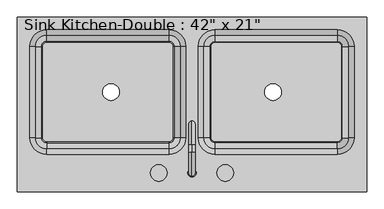
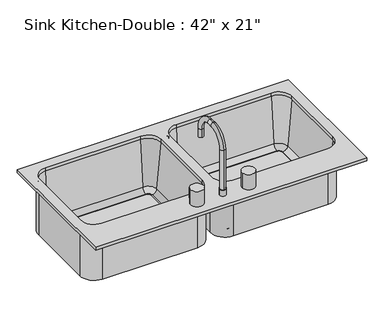
"""IFC4 building model written with IfcOpenShell, lengths in millimetres: flow terminal geometry."""

from ifc_helpers import new_model, si_unit, point, frame, frame_2d, origin, place, context, project, spatial, polyline, circle_curve, ellipse_curve, trimmed, segment, composite_curve, outline, extrude, source, transform, mapped, element, save
from ifc_brep_helpers import plane_surface, cylinder_surface, revolved_surface, advanced_brep


def flow_terminal_7482ecd1(model_context):
    return source(origin(), model_context, "Body", "SolidModel", [
        advanced_brep(
        [(2.9892406, -211.8954011, 927.1), (28.3892406, -211.8954011, 927.1), (15.6892406, -221.4204011, 1114.425), (15.6892406, -221.4204011, 952.5), (15.6892406, -202.3704011, 952.5), (15.6892406, -202.3704011, 1114.425), (15.6892406, -148.3954011, 1168.4), (15.6892406, -148.3954011, 1187.45), (15.6892406, -126.1704011, 1168.4), (15.6892406, -126.1704011, 1187.45), (15.6892406, -72.1954011, 1114.425), (15.6892406, -53.1454011, 1114.425), (15.6892406, -53.1454011, 1079.5), (15.6892406, -72.1954011, 1079.5), (2.9892406, -211.8954011, 952.5), (28.3892406, -211.8954011, 952.5)],
        [
            (0, 1, circle_curve(frame((15.6892406, -211.8954011, 927.1), z_axis=(0.0, 0.0, -1.0), x_axis=(1.0, 0.0, 0.0)), 12.7)),
            (1, 0, circle_curve(frame((15.6892406, -211.8954011, 927.1), z_axis=(0.0, 0.0, -1.0), x_axis=(1.0, 0.0, 0.0)), 12.7)),
            (2, 3),
            (3, 4, circle_curve(frame((15.6892406, -211.8954011, 952.5), z_axis=(0.0, 0.0, 1.0), x_axis=(0.0, 1.0, 0.0)), 9.525)),
            (4, 5),
            (5, 2, circle_curve(frame((15.6892406, -211.8954011, 1114.425), z_axis=(0.0, 0.0, -1.0), x_axis=(0.0, 1.0, 0.0)), 9.525)),
            (4, 3, circle_curve(frame((15.6892406, -211.8954011, 952.5), z_axis=(0.0, 0.0, 1.0), x_axis=(0.0, 1.0, 0.0)), 9.525)),
            (2, 5, circle_curve(frame((15.6892406, -211.8954011, 1114.425), z_axis=(0.0, 0.0, -1.0), x_axis=(0.0, 1.0, 0.0)), 9.525)),
            (5, 6, circle_curve(frame((15.6892406, -148.3954011, 1114.425), z_axis=(-1.0, 0.0, 0.0), x_axis=(0.0, -1.0, 0.0)), 53.975)),
            (6, 7, circle_curve(frame((15.6892406, -148.3954011, 1177.925), z_axis=(0.0, -1.0, 0.0), x_axis=(0.0, 0.0, -1.0)), 9.525)),
            (7, 2, circle_curve(frame((15.6892406, -148.3954011, 1114.425), z_axis=(1.0, 0.0, 0.0), x_axis=(0.0, -1.0, 0.0)), 73.025)),
            (7, 6, circle_curve(frame((15.6892406, -148.3954011, 1177.925), z_axis=(0.0, -1.0, 0.0), x_axis=(0.0, 0.0, -1.0)), 9.525)),
            (6, 8),
            (8, 9, circle_curve(frame((15.6892406, -126.1704011, 1177.925), z_axis=(0.0, -1.0, 0.0), x_axis=(0.0, 0.0, -1.0)), 9.525)),
            (9, 7),
            (9, 8, circle_curve(frame((15.6892406, -126.1704011, 1177.925), z_axis=(0.0, -1.0, 0.0), x_axis=(0.0, 0.0, -1.0)), 9.525)),
            (8, 10, circle_curve(frame((15.6892406, -126.1704011, 1114.425), z_axis=(-1.0, 0.0, 0.0), x_axis=(0.0, 0.0, 1.0)), 53.975)),
            (10, 11, circle_curve(frame((15.6892406, -62.6704011, 1114.425), z_axis=(0.0, 0.0, 1.0), x_axis=(0.0, -1.0, 0.0)), 9.525)),
            (11, 9, circle_curve(frame((15.6892406, -126.1704011, 1114.425), z_axis=(1.0, 0.0, 0.0), x_axis=(0.0, 0.0, 1.0)), 73.025)),
            (11, 10, circle_curve(frame((15.6892406, -62.6704011, 1114.425), z_axis=(0.0, 0.0, 1.0), x_axis=(0.0, -1.0, 0.0)), 9.525)),
            (12, 13, circle_curve(frame((15.6892406, -62.6704011, 1079.5), z_axis=(0.0, 0.0, -1.0), x_axis=(0.0, -1.0, 0.0)), 9.525)),
            (13, 12, circle_curve(frame((15.6892406, -62.6704011, 1079.5), z_axis=(0.0, 0.0, -1.0), x_axis=(0.0, -1.0, 0.0)), 9.525)),
            (10, 13),
            (12, 11),
            (14, 15, circle_curve(frame((15.6892406, -211.8954011, 952.5), z_axis=(0.0, 0.0, 1.0), x_axis=(1.0, 0.0, 0.0)), 12.7)),
            (15, 14, circle_curve(frame((15.6892406, -211.8954011, 952.5), z_axis=(0.0, 0.0, 1.0), x_axis=(1.0, 0.0, 0.0)), 12.7)),
            (15, 1),
            (0, 14),
        ],
        [
            plane_surface(frame((15.6892406, -202.3704011, 927.1), z_axis=(0.0, 0.0, -1.0), x_axis=(1.0, 0.0, 0.0))),
            cylinder_surface(frame((15.6892406, -211.8954011, 927.1), z_axis=(0.0, 0.0, -1.0), x_axis=(0.0, 1.0, 0.0)), 9.525),
            revolved_surface(trimmed(ellipse_curve(frame((15.6892406, -211.8954011, 1114.425), z_axis=(0.0, 0.0, 1.0), x_axis=(0.0, 1.0, 0.0)), 9.525, 9.525), [point((15.6892406, -221.4204011, 1114.425))], [point((15.6892406, -202.3704011, 1114.425))], True, "CARTESIAN"), (15.6892406, -148.3954011, 1114.425), (1.0, 0.0, 0.0)),
            revolved_surface(trimmed(ellipse_curve(frame((15.6892406, -211.8954011, 1114.425), z_axis=(0.0, 0.0, 1.0), x_axis=(0.0, 1.0, 0.0)), 9.525, 9.525), [point((15.6892406, -202.3704011, 1114.425))], [point((15.6892406, -221.4204011, 1114.425))], True, "CARTESIAN"), (15.6892406, -148.3954011, 1114.425), (1.0, 0.0, 0.0)),
            cylinder_surface(frame((15.6892406, -148.3954011, 1177.925), z_axis=(0.0, -1.0, 0.0), x_axis=(0.0, 0.0, -1.0)), 9.525),
            revolved_surface(trimmed(ellipse_curve(frame((15.6892406, -126.1704011, 1177.925), z_axis=(0.0, 1.0, 0.0), x_axis=(0.0, 0.0, -1.0)), 9.525, 9.525), [point((15.6892406, -126.1704011, 1187.45))], [point((15.6892406, -126.1704011, 1168.4))], True, "CARTESIAN"), (15.6892406, -126.1704011, 1114.425), (1.0, 0.0, 0.0)),
            revolved_surface(trimmed(ellipse_curve(frame((15.6892406, -126.1704011, 1177.925), z_axis=(0.0, 1.0, 0.0), x_axis=(0.0, 0.0, -1.0)), 9.525, 9.525), [point((15.6892406, -126.1704011, 1168.4))], [point((15.6892406, -126.1704011, 1187.45))], True, "CARTESIAN"), (15.6892406, -126.1704011, 1114.425), (1.0, 0.0, 0.0)),
            plane_surface(frame((15.6892406, -53.1454011, 1079.5), z_axis=(0.0, 0.0, -1.0), x_axis=(-1.0, 0.0, 0.0))),
            cylinder_surface(frame((15.6892406, -62.6704011, 1114.425), z_axis=(0.0, 0.0, 1.0), x_axis=(0.0, -1.0, 0.0)), 9.525),
            plane_surface(frame((28.3892406, -211.8954011, 952.5), z_axis=(0.0, 0.0, 1.0), x_axis=(0.0, -1.0, 0.0))),
            cylinder_surface(frame((15.6892406, -211.8954011, 927.1), z_axis=(0.0, 0.0, 1.0), x_axis=(1.0, 0.0, 0.0)), 12.7),
        ],
        [
            (0, [[1, 2]]),
            (1, [[3, 4, 5, 6]]),
            (1, [[-5, 7, -3, 8]]),
            (2, [[9, 10, 11, -6]]),
            (3, [[-11, 12, -9, -8]]),
            (4, [[13, 14, 15, -10]]),
            (4, [[-15, 16, -13, -12]]),
            (5, [[17, 18, 19, -14]]),
            (6, [[-19, 20, -17, -16]]),
            (7, [[21, 22]]),
            (8, [[23, -21, 24, -18]]),
            (8, [[-24, -22, -23, -20]]),
            (9, [[25, 26], [-7, -4]]),
            (10, [[27, -1, 28, -26]]),
            (10, [[-28, -2, -27, -25]]),
        ],
    ),
        advanced_brep(
        [(549.0892406, -269.0454011, 927.1), (549.0892406, 264.3545989, 927.1), (-517.7107594, 264.3545989, 927.1), (-517.7107594, -269.0454011, 927.1), (-54.1607594, -154.7454011, 927.1), (-428.8107594, -154.7454011, 927.1), (-479.6107594, -103.9454011, 927.1), (-479.6107594, 175.4545989, 927.1), (-428.8107594, 226.2545989, 927.1), (-54.1607594, 226.2545989, 927.1), (-3.3607594, 175.4545989, 927.1), (-3.3607594, -103.9454011, 927.1), (85.5392406, 226.2545989, 927.1), (460.1892406, 226.2545989, 927.1), (510.9892406, 175.4545989, 927.1), (510.9892406, -103.9454011, 927.1), (460.1892406, -154.7454011, 927.1), (85.5392406, -154.7454011, 927.1), (34.7392406, -103.9454011, 927.1), (34.7392406, 175.4545989, 927.1), (549.0892406, -269.0454011, 914.4), (-517.7107594, -269.0454011, 914.4), (-517.7107594, 264.3545989, 914.4), (549.0892406, 264.3545989, 914.4), (85.5392406, -161.0954011, 914.4), (460.1892406, -161.0954011, 914.4), (517.3392406, -103.9454011, 914.4), (517.3392406, 175.4545989, 914.4), (460.1892406, 232.6045989, 914.4), (85.5392406, 232.6045989, 914.4), (28.3892406, 175.4545989, 914.4), (28.3892406, -103.9454011, 914.4), (2.9892406, -103.9454011, 914.4), (2.9892406, 175.4545989, 914.4), (-54.1607594, 232.6045989, 914.4), (-428.8107594, 232.6045989, 914.4), (-485.9607594, 175.4545989, 914.4), (-485.9607594, -103.9454011, 914.4), (-428.8107594, -161.0954011, 914.4), (-54.1607594, -161.0954011, 914.4), (-3.3607594, -103.9454011, 914.4), (-54.1607594, -154.7454011, 914.4), (-3.3607594, 175.4545989, 914.4), (-54.1607594, 226.2545989, 914.4), (-428.8107594, 226.2545989, 914.4), (-479.6107594, 175.4545989, 914.4), (-479.6107594, -103.9454011, 914.4), (-428.8107594, -154.7454011, 914.4), (34.7392406, 175.4545989, 914.4), (85.5392406, 226.2545989, 914.4), (34.7392406, -103.9454011, 914.4), (85.5392406, -154.7454011, 914.4), (460.1892406, -154.7454011, 914.4), (510.9892406, -103.9454011, 914.4), (510.9892406, 175.4545989, 914.4), (460.1892406, 226.2545989, 914.4), (2.9892406, -103.9454011, 698.5), (-54.1607594, -161.0954011, 698.5), (-54.1607594, -116.6454011, 698.5), (-41.4607594, -103.9454011, 698.5), (-54.1607594, -116.6454011, 708.025), (-41.4607594, -103.9454011, 708.025), (-54.1607594, -119.2338193, 708.025), (-38.8723412, -103.9454011, 708.025), (-54.1607594, -138.2113283, 725.4146831), (-19.8948322, -103.9454011, 725.4146831), (2.9892406, 175.4545989, 698.5), (-41.4607594, 175.4545989, 698.5), (-41.4607594, 175.4545989, 708.025), (-38.8723412, 175.4545989, 708.025), (-19.8948322, 175.4545989, 725.4146831), (-54.1607594, 232.6045989, 698.5), (-54.1607594, 188.1545989, 698.5), (-54.1607594, 188.1545989, 708.025), (-54.1607594, 190.7430171, 708.025), (-54.1607594, 209.7205261, 725.4146831), (-428.8107594, 232.6045989, 698.5), (-428.8107594, 188.1545989, 698.5), (-428.8107594, 188.1545989, 708.025), (-428.8107594, 190.7430171, 708.025), (-428.8107594, 209.7205261, 725.4146831), (-485.9607594, 175.4545989, 698.5), (-441.5107594, 175.4545989, 698.5), (-441.5107594, 175.4545989, 708.025), (-444.0991776, 175.4545989, 708.025), (-463.0766866, 175.4545989, 725.4146831), (-485.9607594, -103.9454011, 698.5), (-441.5107594, -103.9454011, 698.5), (-441.5107594, -103.9454011, 708.025), (-444.0991776, -103.9454011, 708.025), (-463.0766866, -103.9454011, 725.4146831), (-428.8107594, -161.0954011, 698.5), (-428.8107594, -116.6454011, 698.5), (-428.8107594, -116.6454011, 708.025), (-428.8107594, -119.2338193, 708.025), (-428.8107594, -138.2113283, 725.4146831), (51.2733134, -103.9454011, 725.4146831), (85.5392406, -138.2113283, 725.4146831), (85.5392406, -119.2338193, 708.025), (70.2508224, -103.9454011, 708.025), (85.5392406, -116.6454011, 708.025), (72.8392406, -103.9454011, 708.025), (85.5392406, -116.6454011, 698.5), (72.8392406, -103.9454011, 698.5), (85.5392406, -161.0954011, 698.5), (28.3892406, -103.9454011, 698.5), (51.2733134, 175.4545989, 725.4146831), (70.2508224, 175.4545989, 708.025), (72.8392406, 175.4545989, 708.025), (72.8392406, 175.4545989, 698.5), (28.3892406, 175.4545989, 698.5), (85.5392406, 209.7205261, 725.4146831), (85.5392406, 190.7430171, 708.025), (85.5392406, 188.1545989, 708.025), (85.5392406, 188.1545989, 698.5), (85.5392406, 232.6045989, 698.5), (460.1892406, 209.7205261, 725.4146831), (460.1892406, 190.7430171, 708.025), (460.1892406, 188.1545989, 708.025), (460.1892406, 188.1545989, 698.5), (460.1892406, 232.6045989, 698.5), (494.4551678, 175.4545989, 725.4146831), (475.4776588, 175.4545989, 708.025), (472.8892406, 175.4545989, 708.025), (472.8892406, 175.4545989, 698.5), (517.3392406, 175.4545989, 698.5), (494.4551678, -103.9454011, 725.4146831), (475.4776588, -103.9454011, 708.025), (472.8892406, -103.9454011, 708.025), (472.8892406, -103.9454011, 698.5), (517.3392406, -103.9454011, 698.5), (460.1892406, -138.2113283, 725.4146831), (460.1892406, -119.2338193, 708.025), (460.1892406, -116.6454011, 708.025), (460.1892406, -116.6454011, 698.5), (460.1892406, -161.0954011, 698.5)],
        [
            (0, 1),
            (1, 2),
            (2, 3),
            (3, 0),
            (4, 5),
            (5, 6, circle_curve(frame((-428.8107594, -103.9454011, 927.1), z_axis=(0.0, 0.0, -1.0), x_axis=(1.0, 0.0, 0.0)), 50.8)),
            (6, 7),
            (7, 8, circle_curve(frame((-428.8107594, 175.4545989, 927.1), z_axis=(0.0, 0.0, -1.0), x_axis=(1.0, 0.0, 0.0)), 50.8)),
            (8, 9),
            (9, 10, circle_curve(frame((-54.1607594, 175.4545989, 927.1), z_axis=(0.0, 0.0, -1.0), x_axis=(1.0, 0.0, 0.0)), 50.8)),
            (10, 11),
            (11, 4, circle_curve(frame((-54.1607594, -103.9454011, 927.1), z_axis=(0.0, 0.0, -1.0), x_axis=(1.0, 0.0, 0.0)), 50.8)),
            (12, 13),
            (13, 14, circle_curve(frame((460.1892406, 175.4545989, 927.1), z_axis=(0.0, 0.0, -1.0), x_axis=(1.0, 0.0, 0.0)), 50.8)),
            (14, 15),
            (15, 16, circle_curve(frame((460.1892406, -103.9454011, 927.1), z_axis=(0.0, 0.0, -1.0), x_axis=(1.0, 0.0, 0.0)), 50.8)),
            (16, 17),
            (17, 18, circle_curve(frame((85.5392406, -103.9454011, 927.1), z_axis=(0.0, 0.0, -1.0), x_axis=(1.0, 0.0, 0.0)), 50.8)),
            (18, 19),
            (19, 12, circle_curve(frame((85.5392406, 175.4545989, 927.1), z_axis=(0.0, 0.0, -1.0), x_axis=(1.0, 0.0, 0.0)), 50.8)),
            (20, 21),
            (21, 22),
            (22, 23),
            (23, 20),
            (24, 25),
            (25, 26, circle_curve(frame((460.1892406, -103.9454011, 914.4), z_axis=(0.0, 0.0, 1.0), x_axis=(1.0, 0.0, 0.0)), 57.15)),
            (26, 27),
            (27, 28, circle_curve(frame((460.1892406, 175.4545989, 914.4), z_axis=(0.0, 0.0, 1.0), x_axis=(0.0, 1.0, 0.0)), 57.15)),
            (28, 29),
            (29, 30, circle_curve(frame((85.5392406, 175.4545989, 914.4), z_axis=(0.0, 0.0, 1.0), x_axis=(-1.0, 0.0, 0.0)), 57.15)),
            (30, 31),
            (31, 24, circle_curve(frame((85.5392406, -103.9454011, 914.4), z_axis=(0.0, 0.0, 1.0), x_axis=(0.0, -1.0, 0.0)), 57.15)),
            (32, 33),
            (33, 34, circle_curve(frame((-54.1607594, 175.4545989, 914.4), z_axis=(0.0, 0.0, 1.0), x_axis=(1.0, 0.0, 0.0)), 57.15)),
            (34, 35),
            (35, 36, circle_curve(frame((-428.8107594, 175.4545989, 914.4), z_axis=(0.0, 0.0, 1.0), x_axis=(0.0, 1.0, 0.0)), 57.15)),
            (36, 37),
            (37, 38, circle_curve(frame((-428.8107594, -103.9454011, 914.4), z_axis=(0.0, 0.0, 1.0), x_axis=(-1.0, 0.0, 0.0)), 57.15)),
            (38, 39),
            (39, 32, circle_curve(frame((-54.1607594, -103.9454011, 914.4), z_axis=(0.0, 0.0, 1.0), x_axis=(0.0, -1.0, 0.0)), 57.15)),
            (3, 21),
            (20, 0),
            (2, 22),
            (1, 23),
            (11, 40),
            (40, 41, circle_curve(frame((-54.1607594, -103.9454011, 914.4), z_axis=(0.0, 0.0, -1.0), x_axis=(1.0, 0.0, 0.0)), 50.8)),
            (41, 4),
            (10, 42),
            (42, 40),
            (9, 43),
            (43, 42, circle_curve(frame((-54.1607594, 175.4545989, 914.4), z_axis=(0.0, 0.0, -1.0), x_axis=(1.0, 0.0, 0.0)), 50.8)),
            (8, 44),
            (44, 43),
            (7, 45),
            (45, 44, circle_curve(frame((-428.8107594, 175.4545989, 914.4), z_axis=(0.0, 0.0, -1.0), x_axis=(1.0, 0.0, 0.0)), 50.8)),
            (6, 46),
            (46, 45),
            (5, 47),
            (47, 46, circle_curve(frame((-428.8107594, -103.9454011, 914.4), z_axis=(0.0, 0.0, -1.0), x_axis=(1.0, 0.0, 0.0)), 50.8)),
            (41, 47),
            (19, 48),
            (48, 49, circle_curve(frame((85.5392406, 175.4545989, 914.4), z_axis=(0.0, 0.0, -1.0), x_axis=(1.0, 0.0, 0.0)), 50.8)),
            (49, 12),
            (18, 50),
            (50, 48),
            (17, 51),
            (51, 50, circle_curve(frame((85.5392406, -103.9454011, 914.4), z_axis=(0.0, 0.0, -1.0), x_axis=(1.0, 0.0, 0.0)), 50.8)),
            (16, 52),
            (52, 51),
            (15, 53),
            (53, 52, circle_curve(frame((460.1892406, -103.9454011, 914.4), z_axis=(0.0, 0.0, -1.0), x_axis=(1.0, 0.0, 0.0)), 50.8)),
            (14, 54),
            (54, 53),
            (13, 55),
            (55, 54, circle_curve(frame((460.1892406, 175.4545989, 914.4), z_axis=(0.0, 0.0, -1.0), x_axis=(1.0, 0.0, 0.0)), 50.8)),
            (49, 55),
            (56, 32),
            (39, 57),
            (57, 56, circle_curve(frame((-54.1607594, -103.9454011, 698.5), z_axis=(0.0, 0.0, 1.0), x_axis=(0.0, -1.0, 0.0)), 57.15)),
            (57, 58),
            (58, 59, circle_curve(frame((-54.1607594, -103.9454011, 698.5), z_axis=(0.0, 0.0, 1.0), x_axis=(0.0, -1.0, 0.0)), 12.7)),
            (59, 56),
            (58, 60),
            (60, 61, circle_curve(frame((-54.1607594, -103.9454011, 708.025), z_axis=(0.0, 0.0, 1.0), x_axis=(0.0, -1.0, 0.0)), 12.7)),
            (61, 59),
            (60, 62),
            (62, 63, circle_curve(frame((-54.1607594, -103.9454011, 708.025), z_axis=(0.0, 0.0, 1.0), x_axis=(0.0, -1.0, 0.0)), 15.2884182)),
            (63, 61),
            (62, 64, circle_curve(frame((-54.1607594, -119.2338193, 727.075), z_axis=(-1.0, 0.0, 0.0), x_axis=(0.0, -1.0, 0.0)), 19.05)),
            (64, 65, circle_curve(frame((-54.1607594, -103.9454011, 725.4146831), z_axis=(0.0, 0.0, 1.0), x_axis=(0.0, -1.0, 0.0)), 34.2659272)),
            (65, 63, circle_curve(frame((-38.8723412, -103.9454011, 727.075), z_axis=(0.0, 1.0, 0.0), x_axis=(1.0, 0.0, 0.0)), 19.05)),
            (64, 41),
            (40, 65),
            (56, 66),
            (66, 33),
            (59, 67),
            (67, 66),
            (61, 68),
            (68, 67),
            (63, 69),
            (69, 68),
            (65, 70),
            (70, 69, circle_curve(frame((-38.8723412, 175.4545989, 727.075), z_axis=(0.0, 1.0, 0.0), x_axis=(1.0, 0.0, 0.0)), 19.05)),
            (42, 70),
            (66, 71, circle_curve(frame((-54.1607594, 175.4545989, 698.5), z_axis=(0.0, 0.0, 1.0), x_axis=(1.0, 0.0, 0.0)), 57.15)),
            (71, 34),
            (67, 72, circle_curve(frame((-54.1607594, 175.4545989, 698.5), z_axis=(0.0, 0.0, 1.0), x_axis=(1.0, 0.0, 0.0)), 12.7)),
            (72, 71),
            (68, 73, circle_curve(frame((-54.1607594, 175.4545989, 708.025), z_axis=(0.0, 0.0, 1.0), x_axis=(1.0, 0.0, 0.0)), 12.7)),
            (73, 72),
            (69, 74, circle_curve(frame((-54.1607594, 175.4545989, 708.025), z_axis=(0.0, 0.0, 1.0), x_axis=(1.0, 0.0, 0.0)), 15.2884182)),
            (74, 73),
            (70, 75, circle_curve(frame((-54.1607594, 175.4545989, 725.4146831), z_axis=(0.0, 0.0, 1.0), x_axis=(1.0, 0.0, 0.0)), 34.2659272)),
            (75, 74, circle_curve(frame((-54.1607594, 190.7430171, 727.075), z_axis=(-1.0, 0.0, 0.0), x_axis=(0.0, 1.0, 0.0)), 19.05)),
            (43, 75),
            (71, 76),
            (76, 35),
            (72, 77),
            (77, 76),
            (73, 78),
            (78, 77),
            (74, 79),
            (79, 78),
            (75, 80),
            (80, 79, circle_curve(frame((-428.8107594, 190.7430171, 727.075), z_axis=(-1.0, 0.0, 0.0), x_axis=(0.0, 1.0, 0.0)), 19.05)),
            (44, 80),
            (76, 81, circle_curve(frame((-428.8107594, 175.4545989, 698.5), z_axis=(0.0, 0.0, 1.0), x_axis=(0.0, 1.0, 0.0)), 57.15)),
            (81, 36),
            (77, 82, circle_curve(frame((-428.8107594, 175.4545989, 698.5), z_axis=(0.0, 0.0, 1.0), x_axis=(0.0, 1.0, 0.0)), 12.7)),
            (82, 81),
            (78, 83, circle_curve(frame((-428.8107594, 175.4545989, 708.025), z_axis=(0.0, 0.0, 1.0), x_axis=(0.0, 1.0, 0.0)), 12.7)),
            (83, 82),
            (79, 84, circle_curve(frame((-428.8107594, 175.4545989, 708.025), z_axis=(0.0, 0.0, 1.0), x_axis=(0.0, 1.0, 0.0)), 15.2884182)),
            (84, 83),
            (80, 85, circle_curve(frame((-428.8107594, 175.4545989, 725.4146831), z_axis=(0.0, 0.0, 1.0), x_axis=(0.0, 1.0, 0.0)), 34.2659272)),
            (85, 84, circle_curve(frame((-444.0991776, 175.4545989, 727.075), z_axis=(0.0, -1.0, 0.0), x_axis=(-1.0, 0.0, 0.0)), 19.05)),
            (45, 85),
            (81, 86),
            (86, 37),
            (82, 87),
            (87, 86),
            (83, 88),
            (88, 87),
            (84, 89),
            (89, 88),
            (85, 90),
            (90, 89, circle_curve(frame((-444.0991776, -103.9454011, 727.075), z_axis=(0.0, -1.0, 0.0), x_axis=(-1.0, 0.0, 0.0)), 19.05)),
            (46, 90),
            (86, 91, circle_curve(frame((-428.8107594, -103.9454011, 698.5), z_axis=(0.0, 0.0, 1.0), x_axis=(-1.0, 0.0, 0.0)), 57.15)),
            (91, 38),
            (87, 92, circle_curve(frame((-428.8107594, -103.9454011, 698.5), z_axis=(0.0, 0.0, 1.0), x_axis=(-1.0, 0.0, 0.0)), 12.7)),
            (92, 91),
            (88, 93, circle_curve(frame((-428.8107594, -103.9454011, 708.025), z_axis=(0.0, 0.0, 1.0), x_axis=(-1.0, 0.0, 0.0)), 12.7)),
            (93, 92),
            (89, 94, circle_curve(frame((-428.8107594, -103.9454011, 708.025), z_axis=(0.0, 0.0, 1.0), x_axis=(-1.0, 0.0, 0.0)), 15.2884182)),
            (94, 93),
            (90, 95, circle_curve(frame((-428.8107594, -103.9454011, 725.4146831), z_axis=(0.0, 0.0, 1.0), x_axis=(-1.0, 0.0, 0.0)), 34.2659272)),
            (95, 94, circle_curve(frame((-428.8107594, -119.2338193, 727.075), z_axis=(1.0, 0.0, 0.0), x_axis=(0.0, -1.0, 0.0)), 19.05)),
            (47, 95),
            (91, 57),
            (92, 58),
            (93, 60),
            (94, 62),
            (95, 64),
            (96, 50),
            (51, 97),
            (97, 96, circle_curve(frame((85.5392406, -103.9454011, 725.4146831), z_axis=(0.0, 0.0, -1.0), x_axis=(0.0, -1.0, 0.0)), 34.2659272)),
            (97, 98, circle_curve(frame((85.5392406, -119.2338193, 727.075), z_axis=(1.0, 0.0, 0.0), x_axis=(0.0, 1.0, 0.0)), 19.05)),
            (98, 99, circle_curve(frame((85.5392406, -103.9454011, 708.025), z_axis=(0.0, 0.0, -1.0), x_axis=(0.0, -1.0, 0.0)), 15.2884182)),
            (99, 96, circle_curve(frame((70.2508224, -103.9454011, 727.075), z_axis=(0.0, 1.0, 0.0), x_axis=(1.0, 0.0, 0.0)), 19.05)),
            (98, 100),
            (100, 101, circle_curve(frame((85.5392406, -103.9454011, 708.025), z_axis=(0.0, 0.0, -1.0), x_axis=(0.0, -1.0, 0.0)), 12.7)),
            (101, 99),
            (100, 102),
            (102, 103, circle_curve(frame((85.5392406, -103.9454011, 698.5), z_axis=(0.0, 0.0, -1.0), x_axis=(0.0, -1.0, 0.0)), 12.7)),
            (103, 101),
            (102, 104),
            (104, 105, circle_curve(frame((85.5392406, -103.9454011, 698.5), z_axis=(0.0, 0.0, -1.0), x_axis=(0.0, -1.0, 0.0)), 57.15)),
            (105, 103),
            (104, 24),
            (31, 105),
            (96, 106),
            (106, 48),
            (99, 107),
            (107, 106, circle_curve(frame((70.2508224, 175.4545989, 727.075), z_axis=(0.0, 1.0, 0.0), x_axis=(1.0, 0.0, 0.0)), 19.05)),
            (101, 108),
            (108, 107),
            (103, 109),
            (109, 108),
            (105, 110),
            (110, 109),
            (30, 110),
            (106, 111, circle_curve(frame((85.5392406, 175.4545989, 725.4146831), z_axis=(0.0, 0.0, -1.0), x_axis=(-1.0, 0.0, 0.0)), 34.2659272)),
            (111, 49),
            (107, 112, circle_curve(frame((85.5392406, 175.4545989, 708.025), z_axis=(0.0, 0.0, -1.0), x_axis=(-1.0, 0.0, 0.0)), 15.2884182)),
            (112, 111, circle_curve(frame((85.5392406, 190.7430171, 727.075), z_axis=(1.0, 0.0, 0.0), x_axis=(0.0, -1.0, 0.0)), 19.05)),
            (108, 113, circle_curve(frame((85.5392406, 175.4545989, 708.025), z_axis=(0.0, 0.0, -1.0), x_axis=(-1.0, 0.0, 0.0)), 12.7)),
            (113, 112),
            (109, 114, circle_curve(frame((85.5392406, 175.4545989, 698.5), z_axis=(0.0, 0.0, -1.0), x_axis=(-1.0, 0.0, 0.0)), 12.7)),
            (114, 113),
            (110, 115, circle_curve(frame((85.5392406, 175.4545989, 698.5), z_axis=(0.0, 0.0, -1.0), x_axis=(-1.0, 0.0, 0.0)), 57.15)),
            (115, 114),
            (29, 115),
            (111, 116),
            (116, 55),
            (112, 117),
            (117, 116, circle_curve(frame((460.1892406, 190.7430171, 727.075), z_axis=(1.0, 0.0, 0.0), x_axis=(0.0, -1.0, 0.0)), 19.05)),
            (113, 118),
            (118, 117),
            (114, 119),
            (119, 118),
            (115, 120),
            (120, 119),
            (28, 120),
            (116, 121, circle_curve(frame((460.1892406, 175.4545989, 725.4146831), z_axis=(0.0, 0.0, -1.0), x_axis=(0.0, 1.0, 0.0)), 34.2659272)),
            (121, 54),
            (117, 122, circle_curve(frame((460.1892406, 175.4545989, 708.025), z_axis=(0.0, 0.0, -1.0), x_axis=(0.0, 1.0, 0.0)), 15.2884182)),
            (122, 121, circle_curve(frame((475.4776588, 175.4545989, 727.075), z_axis=(0.0, -1.0, 0.0), x_axis=(-1.0, 0.0, 0.0)), 19.05)),
            (118, 123, circle_curve(frame((460.1892406, 175.4545989, 708.025), z_axis=(0.0, 0.0, -1.0), x_axis=(0.0, 1.0, 0.0)), 12.7)),
            (123, 122),
            (119, 124, circle_curve(frame((460.1892406, 175.4545989, 698.5), z_axis=(0.0, 0.0, -1.0), x_axis=(0.0, 1.0, 0.0)), 12.7)),
            (124, 123),
            (120, 125, circle_curve(frame((460.1892406, 175.4545989, 698.5), z_axis=(0.0, 0.0, -1.0), x_axis=(0.0, 1.0, 0.0)), 57.15)),
            (125, 124),
            (27, 125),
            (121, 126),
            (126, 53),
            (122, 127),
            (127, 126, circle_curve(frame((475.4776588, -103.9454011, 727.075), z_axis=(0.0, -1.0, 0.0), x_axis=(-1.0, 0.0, 0.0)), 19.05)),
            (123, 128),
            (128, 127),
            (124, 129),
            (129, 128),
            (125, 130),
            (130, 129),
            (26, 130),
            (126, 131, circle_curve(frame((460.1892406, -103.9454011, 725.4146831), z_axis=(0.0, 0.0, -1.0), x_axis=(1.0, 0.0, 0.0)), 34.2659272)),
            (131, 52),
            (127, 132, circle_curve(frame((460.1892406, -103.9454011, 708.025), z_axis=(0.0, 0.0, -1.0), x_axis=(1.0, 0.0, 0.0)), 15.2884182)),
            (132, 131, circle_curve(frame((460.1892406, -119.2338193, 727.075), z_axis=(-1.0, 0.0, 0.0), x_axis=(0.0, 1.0, 0.0)), 19.05)),
            (128, 133, circle_curve(frame((460.1892406, -103.9454011, 708.025), z_axis=(0.0, 0.0, -1.0), x_axis=(1.0, 0.0, 0.0)), 12.7)),
            (133, 132),
            (129, 134, circle_curve(frame((460.1892406, -103.9454011, 698.5), z_axis=(0.0, 0.0, -1.0), x_axis=(1.0, 0.0, 0.0)), 12.7)),
            (134, 133),
            (130, 135, circle_curve(frame((460.1892406, -103.9454011, 698.5), z_axis=(0.0, 0.0, -1.0), x_axis=(1.0, 0.0, 0.0)), 57.15)),
            (135, 134),
            (25, 135),
            (131, 97),
            (132, 98),
            (133, 100),
            (134, 102),
            (135, 104),
        ],
        [
            plane_surface(frame((-517.7107594, -269.0454011, 927.1), z_axis=(0.0, 0.0, 1.0), x_axis=(-1.0, 0.0, 0.0))),
            plane_surface(frame((-517.7107594, -269.0454011, 914.4), z_axis=(0.0, 0.0, -1.0), x_axis=(1.0, 0.0, 0.0))),
            plane_surface(frame((549.0892406, -269.0454011, 927.1), z_axis=(0.0, -1.0, 0.0), x_axis=(0.0, 0.0, -1.0))),
            plane_surface(frame((-517.7107594, -269.0454011, 927.1), z_axis=(-1.0, 0.0, 0.0), x_axis=(0.0, 0.0, -1.0))),
            plane_surface(frame((-517.7107594, 264.3545989, 927.1), z_axis=(0.0, 1.0, 0.0), x_axis=(0.0, 0.0, -1.0))),
            plane_surface(frame((549.0892406, 264.3545989, 927.1), z_axis=(1.0, 0.0, 0.0), x_axis=(0.0, 0.0, -1.0))),
            revolved_surface(polyline([(-3.3607594000000063, -103.9454011, 914.4), (-3.3607594000000063, -103.9454011, 927.1)]), (-54.1607594, -103.9454011, 0.0), (0.0, 0.0, -1.0)),
            plane_surface(frame((-3.3607594, -103.9454011, 927.1), z_axis=(-1.0, 0.0, 0.0), x_axis=(0.0, 0.0, -1.0))),
            revolved_surface(polyline([(-3.3607594000000063, 175.4545989, 914.4), (-3.3607594000000063, 175.4545989, 927.1)]), (-54.1607594, 175.4545989, 0.0), (0.0, 0.0, -1.0)),
            plane_surface(frame((-54.1607594, 226.2545989, 927.1), z_axis=(0.0, -1.0, 0.0), x_axis=(0.0, 0.0, -1.0))),
            revolved_surface(polyline([(-378.0107594, 175.4545989, 914.4), (-378.0107594, 175.4545989, 927.1)]), (-428.8107594, 175.4545989, 0.0), (0.0, 0.0, -1.0)),
            plane_surface(frame((-479.6107594, 175.4545989, 927.1), z_axis=(1.0, 0.0, 0.0), x_axis=(0.0, 0.0, -1.0))),
            revolved_surface(polyline([(-378.0107594, -103.9454011, 914.4), (-378.0107594, -103.9454011, 927.1)]), (-428.8107594, -103.9454011, 0.0), (0.0, 0.0, -1.0)),
            plane_surface(frame((-428.8107594, -154.7454011, 927.1), z_axis=(0.0, 1.0, 0.0), x_axis=(0.0, 0.0, -1.0))),
            revolved_surface(polyline([(136.33924059999998, 175.4545989, 914.4), (136.33924059999998, 175.4545989, 927.1)]), (85.5392406, 175.4545989, 0.0), (0.0, 0.0, -1.0)),
            plane_surface(frame((34.7392406, 175.4545989, 927.1), z_axis=(1.0, 0.0, 0.0), x_axis=(0.0, 0.0, -1.0))),
            revolved_surface(polyline([(136.33924059999998, -103.9454011, 914.4), (136.33924059999998, -103.9454011, 927.1)]), (85.5392406, -103.9454011, 0.0), (0.0, 0.0, -1.0)),
            plane_surface(frame((85.5392406, -154.7454011, 927.1), z_axis=(0.0, 1.0, 0.0), x_axis=(0.0, 0.0, -1.0))),
            revolved_surface(polyline([(510.9892406, -103.9454011, 914.4), (510.9892406, -103.9454011, 927.1)]), (460.1892406, -103.9454011, 0.0), (0.0, 0.0, -1.0)),
            plane_surface(frame((510.9892406, -103.9454011, 927.1), z_axis=(-1.0, 0.0, 0.0), x_axis=(0.0, 0.0, -1.0))),
            revolved_surface(polyline([(510.9892406, 175.4545989, 914.4), (510.9892406, 175.4545989, 927.1)]), (460.1892406, 175.4545989, 0.0), (0.0, 0.0, -1.0)),
            plane_surface(frame((460.1892406, 226.2545989, 927.1), z_axis=(0.0, -1.0, 0.0), x_axis=(0.0, 0.0, -1.0))),
            cylinder_surface(frame((-54.1607594, -103.9454011, 0.0), z_axis=(0.0, 0.0, -1.0), x_axis=(0.0, -1.0, 0.0)), 57.15),
            plane_surface(frame((-54.1607594, -103.9454011, 698.5), z_axis=(0.0, 0.0, -1.0), x_axis=(0.0, -1.0, 0.0))),
            revolved_surface(polyline([(-54.1607594, -116.6454011, 698.5), (-54.1607594, -116.6454011, 708.025)]), (-54.1607594, -103.9454011, 0.0), (0.0, 0.0, -1.0)),
            plane_surface(frame((-54.1607594, -103.9454011, 708.025), z_axis=(0.0, 0.0, 1.0), x_axis=(0.0, -1.0, 0.0))),
            revolved_surface(trimmed(ellipse_curve(frame((-54.1607594, -119.2338193, 727.075), z_axis=(-1.0, 0.0, 0.0), x_axis=(0.0, -1.0, 0.0)), 19.05, 19.05), [point((-54.1607594, -119.2338193, 708.025))], [point((-54.1607594, -138.2113283, 725.4146831))], True, "CARTESIAN"), (-54.1607594, -103.9454011, 0.0), (0.0, 0.0, -1.0)),
            revolved_surface(polyline([(-54.1607594, -138.2113283, 725.4146831), (-54.1607594, -154.7454011, 914.4)]), (-54.1607594, -103.9454011, 0.0), (0.0, 0.0, -1.0)),
            plane_surface(frame((2.9892406, -103.9454011, 914.4), z_axis=(1.0, 0.0, 0.0), x_axis=(0.0, 1.0, 0.0))),
            plane_surface(frame((2.9892406, -103.9454011, 698.5), z_axis=(0.0, 0.0, -1.0), x_axis=(0.0, 1.0, 0.0))),
            plane_surface(frame((-41.4607594, -103.9454011, 698.5), z_axis=(-1.0, 0.0, 0.0), x_axis=(0.0, 1.0, 0.0))),
            plane_surface(frame((-41.4607594, -103.9454011, 708.025), z_axis=(0.0, 0.0, 1.0), x_axis=(0.0, 1.0, 0.0))),
            revolved_surface(polyline([(-19.8223412, 175.45459889999998, 727.075), (-19.8223412, -103.9454011, 727.075)]), (-38.8723412, -103.9454011, 727.075), (0.0, 1.0, 0.0)),
            plane_surface(frame((-19.8948322, -103.9454011, 725.4146831), z_axis=(-0.9961946980917439, 0.0, 0.08715574274767722), x_axis=(0.0, 1.0, 0.0))),
            cylinder_surface(frame((-54.1607594, 175.4545989, 0.0), z_axis=(0.0, 0.0, -1.0), x_axis=(1.0, 0.0, 0.0)), 57.15),
            plane_surface(frame((-54.1607594, 175.4545989, 698.5), z_axis=(0.0, 0.0, -1.0), x_axis=(1.0, 0.0, 0.0))),
            revolved_surface(polyline([(-41.4607594, 175.4545989, 698.5), (-41.4607594, 175.4545989, 708.025)]), (-54.1607594, 175.4545989, 0.0), (0.0, 0.0, -1.0)),
            plane_surface(frame((-54.1607594, 175.4545989, 708.025), z_axis=(0.0, 0.0, 1.0), x_axis=(1.0, 0.0, 0.0))),
            revolved_surface(trimmed(ellipse_curve(frame((-38.8723412, 175.4545989, 727.075), z_axis=(0.0, -1.0, 0.0), x_axis=(1.0, 0.0, 0.0)), 19.05, 19.05), [point((-38.8723412, 175.4545989, 708.025))], [point((-19.8948322, 175.4545989, 725.4146831))], True, "CARTESIAN"), (-54.1607594, 175.4545989, 0.0), (0.0, 0.0, -1.0)),
            revolved_surface(polyline([(-19.8948322, 175.4545989, 725.4146831), (-3.3607594, 175.4545989, 914.4)]), (-54.1607594, 175.4545989, 0.0), (0.0, 0.0, -1.0)),
            plane_surface(frame((-54.1607594, 232.6045989, 914.4), z_axis=(0.0, 1.0, 0.0), x_axis=(-1.0, 0.0, 0.0))),
            plane_surface(frame((-54.1607594, 232.6045989, 698.5), z_axis=(0.0, 0.0, -1.0), x_axis=(-1.0, 0.0, 0.0))),
            plane_surface(frame((-54.1607594, 188.1545989, 698.5), z_axis=(0.0, -1.0, 0.0), x_axis=(-1.0, 0.0, 0.0))),
            plane_surface(frame((-54.1607594, 188.1545989, 708.025), z_axis=(0.0, 0.0, 1.0), x_axis=(-1.0, 0.0, 0.0))),
            revolved_surface(polyline([(-428.8107594, 209.79301710000001, 727.075), (-54.1607594, 209.79301710000001, 727.075)]), (-54.1607594, 190.7430171, 727.075), (-1.0, 0.0, 0.0)),
            plane_surface(frame((-54.1607594, 209.7205261, 725.4146831), z_axis=(0.0, -0.9961946980917439, 0.08715574274767722), x_axis=(-1.0, 0.0, 0.0))),
            cylinder_surface(frame((-428.8107594, 175.4545989, 0.0), z_axis=(0.0, 0.0, -1.0), x_axis=(0.0, 1.0, 0.0)), 57.15),
            plane_surface(frame((-428.8107594, 175.4545989, 698.5), z_axis=(0.0, 0.0, -1.0), x_axis=(0.0, 1.0, 0.0))),
            revolved_surface(polyline([(-428.8107594, 188.1545989, 698.5), (-428.8107594, 188.1545989, 708.025)]), (-428.8107594, 175.4545989, 0.0), (0.0, 0.0, -1.0)),
            plane_surface(frame((-428.8107594, 175.4545989, 708.025), z_axis=(0.0, 0.0, 1.0), x_axis=(0.0, 1.0, 0.0))),
            revolved_surface(trimmed(ellipse_curve(frame((-428.8107594, 190.7430171, 727.075), z_axis=(1.0, 0.0, 0.0), x_axis=(0.0, 1.0, 0.0)), 19.05, 19.05), [point((-428.8107594, 190.7430171, 708.025))], [point((-428.8107594, 209.7205261, 725.4146831))], True, "CARTESIAN"), (-428.8107594, 175.4545989, 0.0), (0.0, 0.0, -1.0)),
            revolved_surface(polyline([(-428.8107594, 209.7205261, 725.4146831), (-428.8107594, 226.2545989, 914.4)]), (-428.8107594, 175.4545989, 0.0), (0.0, 0.0, -1.0)),
            plane_surface(frame((-485.9607594, 175.4545989, 914.4), z_axis=(-1.0, 0.0, 0.0), x_axis=(0.0, -1.0, 0.0))),
            plane_surface(frame((-485.9607594, 175.4545989, 698.5), z_axis=(0.0, 0.0, -1.0), x_axis=(0.0, -1.0, 0.0))),
            plane_surface(frame((-441.5107594, 175.4545989, 698.5), z_axis=(1.0, 0.0, 0.0), x_axis=(0.0, -1.0, 0.0))),
            plane_surface(frame((-441.5107594, 175.4545989, 708.025), z_axis=(0.0, 0.0, 1.0), x_axis=(0.0, -1.0, 0.0))),
            revolved_surface(polyline([(-463.14917760000003, -103.94540109999997, 727.075), (-463.14917760000003, 175.4545989, 727.075)]), (-444.0991776, 175.4545989, 727.075), (0.0, -1.0, 0.0)),
            plane_surface(frame((-463.0766866, 175.4545989, 725.4146831), z_axis=(0.9961946980917439, 0.0, 0.08715574274767722), x_axis=(0.0, -1.0, 0.0))),
            cylinder_surface(frame((-428.8107594, -103.9454011, 0.0), z_axis=(0.0, 0.0, -1.0), x_axis=(-1.0, 0.0, 0.0)), 57.15),
            plane_surface(frame((-428.8107594, -103.9454011, 698.5), z_axis=(0.0, 0.0, -1.0), x_axis=(-1.0, 0.0, 0.0))),
            revolved_surface(polyline([(-441.5107594, -103.9454011, 698.5), (-441.5107594, -103.9454011, 708.025)]), (-428.8107594, -103.9454011, 0.0), (0.0, 0.0, -1.0)),
            plane_surface(frame((-428.8107594, -103.9454011, 708.025), z_axis=(0.0, 0.0, 1.0), x_axis=(-1.0, 0.0, 0.0))),
            revolved_surface(trimmed(ellipse_curve(frame((-444.0991776, -103.9454011, 727.075), z_axis=(0.0, 1.0, 0.0), x_axis=(-1.0, 0.0, 0.0)), 19.05, 19.05), [point((-444.0991776, -103.9454011, 708.025))], [point((-463.0766866, -103.9454011, 725.4146831))], True, "CARTESIAN"), (-428.8107594, -103.9454011, 0.0), (0.0, 0.0, -1.0)),
            revolved_surface(polyline([(-463.0766866, -103.9454011, 725.4146831), (-479.6107594, -103.9454011, 914.4)]), (-428.8107594, -103.9454011, 0.0), (0.0, 0.0, -1.0)),
            plane_surface(frame((-428.8107594, -161.0954011, 914.4), z_axis=(0.0, -1.0, 0.0), x_axis=(1.0, 0.0, 0.0))),
            plane_surface(frame((-428.8107594, -161.0954011, 698.5), z_axis=(0.0, 0.0, -1.0), x_axis=(1.0, 0.0, 0.0))),
            plane_surface(frame((-428.8107594, -116.6454011, 698.5), z_axis=(0.0, 1.0, 0.0), x_axis=(1.0, 0.0, 0.0))),
            plane_surface(frame((-428.8107594, -116.6454011, 708.025), z_axis=(0.0, 0.0, 1.0), x_axis=(1.0, 0.0, 0.0))),
            revolved_surface(polyline([(-54.16075940000002, -138.2838193, 727.075), (-428.8107594, -138.2838193, 727.075)]), (-428.8107594, -119.2338193, 727.075), (1.0, 0.0, 0.0)),
            plane_surface(frame((-428.8107594, -138.2113283, 725.4146831), z_axis=(0.0, 0.9961946980917439, 0.08715574274767722), x_axis=(1.0, 0.0, 0.0))),
            revolved_surface(polyline([(85.5392406, -154.7454011, 914.4), (85.5392406, -138.2113283, 725.4146831)]), (85.5392406, -103.9454011, 0.0), (0.0, 0.0, 1.0)),
            revolved_surface(trimmed(ellipse_curve(frame((85.5392406, -119.2338193, 727.075), z_axis=(1.0, 0.0, 0.0), x_axis=(0.0, 1.0, 0.0)), 19.05, 19.05), [point((85.5392406, -138.2113283, 725.4146831))], [point((85.5392406, -119.2338193, 708.025))], True, "CARTESIAN"), (85.5392406, -103.9454011, 0.0), (0.0, 0.0, 1.0)),
            plane_surface(frame((85.5392406, -103.9454011, 708.025), z_axis=(0.0, 0.0, 1.0), x_axis=(0.0, -1.0, 0.0))),
            revolved_surface(polyline([(85.5392406, -116.6454011, 708.025), (85.5392406, -116.6454011, 698.5)]), (85.5392406, -103.9454011, 0.0), (0.0, 0.0, 1.0)),
            plane_surface(frame((85.5392406, -103.9454011, 698.5), z_axis=(0.0, 0.0, -1.0), x_axis=(0.0, -1.0, 0.0))),
            cylinder_surface(frame((85.5392406, -103.9454011, 0.0), z_axis=(0.0, 0.0, 1.0), x_axis=(0.0, -1.0, 0.0)), 57.15),
            plane_surface(frame((34.7392406, -103.9454011, 914.4), z_axis=(0.996194698091745, 0.0, 0.08715574274766508), x_axis=(0.0, 1.0, 0.0))),
            revolved_surface(polyline([(89.3008224, 175.45459889999998, 727.075), (89.3008224, -103.9454011, 727.075)]), (70.2508224, -103.9454011, 727.075), (0.0, 1.0, 0.0)),
            plane_surface(frame((70.2508224, -103.9454011, 708.025), z_axis=(0.0, 0.0, 1.0), x_axis=(0.0, 1.0, 0.0))),
            plane_surface(frame((72.8392406, -103.9454011, 708.025), z_axis=(1.0, 0.0, 0.0), x_axis=(0.0, 1.0, 0.0))),
            plane_surface(frame((72.8392406, -103.9454011, 698.5), z_axis=(0.0, 0.0, -1.0), x_axis=(0.0, 1.0, 0.0))),
            plane_surface(frame((28.3892406, -103.9454011, 698.5), z_axis=(-1.0, 0.0, 0.0), x_axis=(0.0, 1.0, 0.0))),
            revolved_surface(polyline([(34.7392406, 175.4545989, 914.4), (51.2733134, 175.4545989, 725.4146831)]), (85.5392406, 175.4545989, 0.0), (0.0, 0.0, 1.0)),
            revolved_surface(trimmed(ellipse_curve(frame((70.2508224, 175.4545989, 727.075), z_axis=(0.0, -1.0, 0.0), x_axis=(1.0, 0.0, 0.0)), 19.05, 19.05), [point((51.2733134, 175.4545989, 725.4146831))], [point((70.2508224, 175.4545989, 708.025))], True, "CARTESIAN"), (85.5392406, 175.4545989, 0.0), (0.0, 0.0, 1.0)),
            plane_surface(frame((85.5392406, 175.4545989, 708.025), z_axis=(0.0, 0.0, 1.0), x_axis=(-1.0, 0.0, 0.0))),
            revolved_surface(polyline([(72.8392406, 175.4545989, 708.025), (72.8392406, 175.4545989, 698.5)]), (85.5392406, 175.4545989, 0.0), (0.0, 0.0, 1.0)),
            plane_surface(frame((85.5392406, 175.4545989, 698.5), z_axis=(0.0, 0.0, -1.0), x_axis=(-1.0, 0.0, 0.0))),
            cylinder_surface(frame((85.5392406, 175.4545989, 0.0), z_axis=(0.0, 0.0, 1.0), x_axis=(-1.0, 0.0, 0.0)), 57.15),
            plane_surface(frame((85.5392406, 226.2545989, 914.4), z_axis=(0.0, -0.996194698091745, 0.08715574274766508), x_axis=(1.0, 0.0, 0.0))),
            revolved_surface(polyline([(460.18924059999995, 171.6930171, 727.075), (85.5392406, 171.6930171, 727.075)]), (85.5392406, 190.7430171, 727.075), (1.0, 0.0, 0.0)),
            plane_surface(frame((85.5392406, 190.7430171, 708.025), z_axis=(0.0, 0.0, 1.0), x_axis=(1.0, 0.0, 0.0))),
            plane_surface(frame((85.5392406, 188.1545989, 708.025), z_axis=(0.0, -1.0, 0.0), x_axis=(1.0, 0.0, 0.0))),
            plane_surface(frame((85.5392406, 188.1545989, 698.5), z_axis=(0.0, 0.0, -1.0), x_axis=(1.0, 0.0, 0.0))),
            plane_surface(frame((85.5392406, 232.6045989, 698.5), z_axis=(0.0, 1.0, 0.0), x_axis=(1.0, 0.0, 0.0))),
            revolved_surface(polyline([(460.1892406, 226.2545989, 914.4), (460.1892406, 209.7205261, 725.4146831)]), (460.1892406, 175.4545989, 0.0), (0.0, 0.0, 1.0)),
            revolved_surface(trimmed(ellipse_curve(frame((460.1892406, 190.7430171, 727.075), z_axis=(-1.0, 0.0, 0.0), x_axis=(0.0, -1.0, 0.0)), 19.05, 19.05), [point((460.1892406, 209.7205261, 725.4146831))], [point((460.1892406, 190.7430171, 708.025))], True, "CARTESIAN"), (460.1892406, 175.4545989, 0.0), (0.0, 0.0, 1.0)),
            plane_surface(frame((460.1892406, 175.4545989, 708.025), z_axis=(0.0, 0.0, 1.0), x_axis=(0.0, 1.0, 0.0))),
            revolved_surface(polyline([(460.1892406, 188.1545989, 708.025), (460.1892406, 188.1545989, 698.5)]), (460.1892406, 175.4545989, 0.0), (0.0, 0.0, 1.0)),
            plane_surface(frame((460.1892406, 175.4545989, 698.5), z_axis=(0.0, 0.0, -1.0), x_axis=(0.0, 1.0, 0.0))),
            cylinder_surface(frame((460.1892406, 175.4545989, 0.0), z_axis=(0.0, 0.0, 1.0), x_axis=(0.0, 1.0, 0.0)), 57.15),
            plane_surface(frame((510.9892406, 175.4545989, 914.4), z_axis=(-0.996194698091745, 0.0, 0.08715574274766508), x_axis=(0.0, -1.0, 0.0))),
            revolved_surface(polyline([(456.42765879999996, -103.94540109999997, 727.075), (456.42765879999996, 175.4545989, 727.075)]), (475.4776588, 175.4545989, 727.075), (0.0, -1.0, 0.0)),
            plane_surface(frame((475.4776588, 175.4545989, 708.025), z_axis=(0.0, 0.0, 1.0), x_axis=(0.0, -1.0, 0.0))),
            plane_surface(frame((472.8892406, 175.4545989, 708.025), z_axis=(-1.0, 0.0, 0.0), x_axis=(0.0, -1.0, 0.0))),
            plane_surface(frame((472.8892406, 175.4545989, 698.5), z_axis=(0.0, 0.0, -1.0), x_axis=(0.0, -1.0, 0.0))),
            plane_surface(frame((517.3392406, 175.4545989, 698.5), z_axis=(1.0, 0.0, 0.0), x_axis=(0.0, -1.0, 0.0))),
            revolved_surface(polyline([(510.9892406, -103.9454011, 914.4), (494.4551678, -103.9454011, 725.4146831)]), (460.1892406, -103.9454011, 0.0), (0.0, 0.0, 1.0)),
            revolved_surface(trimmed(ellipse_curve(frame((475.4776588, -103.9454011, 727.075), z_axis=(0.0, 1.0, 0.0), x_axis=(-1.0, 0.0, 0.0)), 19.05, 19.05), [point((494.4551678, -103.9454011, 725.4146831))], [point((475.4776588, -103.9454011, 708.025))], True, "CARTESIAN"), (460.1892406, -103.9454011, 0.0), (0.0, 0.0, 1.0)),
            plane_surface(frame((460.1892406, -103.9454011, 708.025), z_axis=(0.0, 0.0, 1.0), x_axis=(1.0, 0.0, 0.0))),
            revolved_surface(polyline([(472.8892406, -103.9454011, 708.025), (472.8892406, -103.9454011, 698.5)]), (460.1892406, -103.9454011, 0.0), (0.0, 0.0, 1.0)),
            plane_surface(frame((460.1892406, -103.9454011, 698.5), z_axis=(0.0, 0.0, -1.0), x_axis=(1.0, 0.0, 0.0))),
            cylinder_surface(frame((460.1892406, -103.9454011, 0.0), z_axis=(0.0, 0.0, 1.0), x_axis=(1.0, 0.0, 0.0)), 57.15),
            plane_surface(frame((460.1892406, -154.7454011, 914.4), z_axis=(0.0, 0.996194698091745, 0.08715574274766508), x_axis=(-1.0, 0.0, 0.0))),
            revolved_surface(polyline([(85.53924060000003, -100.1838193, 727.075), (460.1892406, -100.1838193, 727.075)]), (460.1892406, -119.2338193, 727.075), (-1.0, 0.0, 0.0)),
            plane_surface(frame((460.1892406, -119.2338193, 708.025), z_axis=(0.0, 0.0, 1.0), x_axis=(-1.0, 0.0, 0.0))),
            plane_surface(frame((460.1892406, -116.6454011, 708.025), z_axis=(0.0, 1.0, 0.0), x_axis=(-1.0, 0.0, 0.0))),
            plane_surface(frame((460.1892406, -116.6454011, 698.5), z_axis=(0.0, 0.0, -1.0), x_axis=(-1.0, 0.0, 0.0))),
            plane_surface(frame((460.1892406, -161.0954011, 698.5), z_axis=(0.0, -1.0, 0.0), x_axis=(-1.0, 0.0, 0.0))),
        ],
        [
            (0, [[1, 2, 3, 4], [5, 6, 7, 8, 9, 10, 11, 12], [13, 14, 15, 16, 17, 18, 19, 20]]),
            (1, [[21, 22, 23, 24], [25, 26, 27, 28, 29, 30, 31, 32], [33, 34, 35, 36, 37, 38, 39, 40]]),
            (2, [[41, -21, 42, -4]]),
            (3, [[43, -22, -41, -3]]),
            (4, [[44, -23, -43, -2]]),
            (5, [[-42, -24, -44, -1]]),
            (6, [[45, 46, 47, -12]]),
            (7, [[48, 49, -45, -11]]),
            (8, [[50, 51, -48, -10]]),
            (9, [[52, 53, -50, -9]]),
            (10, [[54, 55, -52, -8]]),
            (11, [[56, 57, -54, -7]]),
            (12, [[58, 59, -56, -6]]),
            (13, [[-47, 60, -58, -5]]),
            (14, [[61, 62, 63, -20]]),
            (15, [[64, 65, -61, -19]]),
            (16, [[66, 67, -64, -18]]),
            (17, [[68, 69, -66, -17]]),
            (18, [[70, 71, -68, -16]]),
            (19, [[72, 73, -70, -15]]),
            (20, [[74, 75, -72, -14]]),
            (21, [[-63, 76, -74, -13]]),
            (22, [[77, -40, 78, 79]]),
            (23, [[80, 81, 82, -79]]),
            (24, [[83, 84, 85, -81]]),
            (25, [[86, 87, 88, -84]]),
            (26, [[89, 90, 91, -87]]),
            (27, [[92, -46, 93, -90]]),
            (28, [[94, 95, -33, -77]]),
            (29, [[96, 97, -94, -82]]),
            (30, [[98, 99, -96, -85]]),
            (31, [[100, 101, -98, -88]]),
            (32, [[102, 103, -100, -91]]),
            (33, [[-49, 104, -102, -93]]),
            (34, [[105, 106, -34, -95]]),
            (35, [[107, 108, -105, -97]]),
            (36, [[109, 110, -107, -99]]),
            (37, [[111, 112, -109, -101]]),
            (38, [[113, 114, -111, -103]]),
            (39, [[-51, 115, -113, -104]]),
            (40, [[116, 117, -35, -106]]),
            (41, [[118, 119, -116, -108]]),
            (42, [[120, 121, -118, -110]]),
            (43, [[122, 123, -120, -112]]),
            (44, [[124, 125, -122, -114]]),
            (45, [[-53, 126, -124, -115]]),
            (46, [[127, 128, -36, -117]]),
            (47, [[129, 130, -127, -119]]),
            (48, [[131, 132, -129, -121]]),
            (49, [[133, 134, -131, -123]]),
            (50, [[135, 136, -133, -125]]),
            (51, [[-55, 137, -135, -126]]),
            (52, [[138, 139, -37, -128]]),
            (53, [[140, 141, -138, -130]]),
            (54, [[142, 143, -140, -132]]),
            (55, [[144, 145, -142, -134]]),
            (56, [[146, 147, -144, -136]]),
            (57, [[-57, 148, -146, -137]]),
            (58, [[149, 150, -38, -139]]),
            (59, [[151, 152, -149, -141]]),
            (60, [[153, 154, -151, -143]]),
            (61, [[155, 156, -153, -145]]),
            (62, [[157, 158, -155, -147]]),
            (63, [[-59, 159, -157, -148]]),
            (64, [[-39, -150, 160, -78]]),
            (65, [[-160, -152, 161, -80]]),
            (66, [[-161, -154, 162, -83]]),
            (67, [[-162, -156, 163, -86]]),
            (68, [[-163, -158, 164, -89]]),
            (69, [[-164, -159, -60, -92]]),
            (70, [[165, -67, 166, 167]]),
            (71, [[168, 169, 170, -167]]),
            (72, [[171, 172, 173, -169]]),
            (73, [[174, 175, 176, -172]]),
            (74, [[177, 178, 179, -175]]),
            (75, [[180, -32, 181, -178]]),
            (76, [[182, 183, -65, -165]]),
            (77, [[184, 185, -182, -170]]),
            (78, [[186, 187, -184, -173]]),
            (79, [[188, 189, -186, -176]]),
            (80, [[190, 191, -188, -179]]),
            (81, [[-31, 192, -190, -181]]),
            (82, [[193, 194, -62, -183]]),
            (83, [[195, 196, -193, -185]]),
            (84, [[197, 198, -195, -187]]),
            (85, [[199, 200, -197, -189]]),
            (86, [[201, 202, -199, -191]]),
            (87, [[-30, 203, -201, -192]]),
            (88, [[204, 205, -76, -194]]),
            (89, [[206, 207, -204, -196]]),
            (90, [[208, 209, -206, -198]]),
            (91, [[210, 211, -208, -200]]),
            (92, [[212, 213, -210, -202]]),
            (93, [[-29, 214, -212, -203]]),
            (94, [[215, 216, -75, -205]]),
            (95, [[217, 218, -215, -207]]),
            (96, [[219, 220, -217, -209]]),
            (97, [[221, 222, -219, -211]]),
            (98, [[223, 224, -221, -213]]),
            (99, [[-28, 225, -223, -214]]),
            (100, [[226, 227, -73, -216]]),
            (101, [[228, 229, -226, -218]]),
            (102, [[230, 231, -228, -220]]),
            (103, [[232, 233, -230, -222]]),
            (104, [[234, 235, -232, -224]]),
            (105, [[-27, 236, -234, -225]]),
            (106, [[237, 238, -71, -227]]),
            (107, [[239, 240, -237, -229]]),
            (108, [[241, 242, -239, -231]]),
            (109, [[243, 244, -241, -233]]),
            (110, [[245, 246, -243, -235]]),
            (111, [[-26, 247, -245, -236]]),
            (112, [[-69, -238, 248, -166]]),
            (113, [[-248, -240, 249, -168]]),
            (114, [[-249, -242, 250, -171]]),
            (115, [[-250, -244, 251, -174]]),
            (116, [[-251, -246, 252, -177]]),
            (117, [[-252, -247, -25, -180]]),
        ],
    ),
        extrude(outline(composite_curve([segment(polyline([(460.1892406, -119.2338193), (85.5392406, -119.2338193)]), True, "CONTINUOUS"), segment(trimmed(circle_curve(frame_2d((85.5392406, -106.5338193)), 12.7), [point((85.5392406, -119.2338193))], [point((72.8392406, -106.5338193))], False, "CARTESIAN"), True, "CONTINUOUS"), segment(polyline([(72.8392406, -106.5338193), (72.8392406, 175.4545989)]), True, "CONTINUOUS"), segment(trimmed(circle_curve(frame_2d((85.5392406, 175.4545989)), 12.7), [point((72.8392406, 175.4545989))], [point((85.5392406, 188.1545989))], False, "CARTESIAN"), True, "CONTINUOUS"), segment(polyline([(85.5392406, 188.1545989), (460.1892406, 188.1545989)]), True, "CONTINUOUS"), segment(trimmed(circle_curve(frame_2d((460.1892406, 175.4545989)), 12.7), [point((460.1892406, 188.1545989))], [point((472.8892406, 175.4545989))], False, "CARTESIAN"), True, "CONTINUOUS"), segment(polyline([(472.8892406, 175.4545989), (472.8892406, -106.5338193)]), True, "CONTINUOUS"), segment(trimmed(circle_curve(frame_2d((460.1892406, -106.5338193)), 12.7), [point((472.8892406, -106.5338193))], [point((460.1892406, -119.2338193))], False, "CARTESIAN"), True, "CONTINUOUS")], self_intersect=False), holes=[composite_curve([segment(trimmed(circle_curve(frame_2d((263.3392406, 35.7545989)), 25.4), [point((237.9392406, 35.7545989))], [point((288.7392406, 35.7545989))], True, "CARTESIAN"), True, "CONTINUOUS"), segment(trimmed(circle_curve(frame_2d((263.3392406, 35.7545989)), 25.4), [point((288.7392406, 35.7545989))], [point((237.9392406, 35.7545989))], True, "CARTESIAN"), True, "CONTINUOUS")], self_intersect=False)]), frame((0.0, 0.0, 698.5), z_axis=(0.0, 0.0, 1.0), x_axis=(1.0, 0.0, 0.0)), (0.0, 0.0, 1.0), 9.525),
        extrude(outline(composite_curve([segment(trimmed(circle_curve(frame_2d((-85.9107594, -211.8954011)), 25.4), [point((-111.3107594, -211.8954011))], [point((-60.5107594, -211.8954011))], False, "CARTESIAN"), True, "CONTINUOUS"), segment(trimmed(circle_curve(frame_2d((-85.9107594, -211.8954011)), 25.4), [point((-60.5107594, -211.8954011))], [point((-111.3107594, -211.8954011))], False, "CARTESIAN"), True, "CONTINUOUS")], self_intersect=False)), frame((0.0, 0.0, 927.1), z_axis=(0.0, 0.0, 1.0), x_axis=(1.0, 0.0, 0.0)), (0.0, 0.0, 1.0), 63.5),
        extrude(outline(composite_curve([segment(trimmed(circle_curve(frame_2d((117.2892406, -211.8954011)), 25.4), [point((91.8892406, -211.8954011))], [point((142.6892406, -211.8954011))], False, "CARTESIAN"), True, "CONTINUOUS"), segment(trimmed(circle_curve(frame_2d((117.2892406, -211.8954011)), 25.4), [point((142.6892406, -211.8954011))], [point((91.8892406, -211.8954011))], False, "CARTESIAN"), True, "CONTINUOUS")], self_intersect=False)), frame((0.0, 0.0, 927.1), z_axis=(0.0, 0.0, 1.0), x_axis=(1.0, 0.0, 0.0)), (0.0, 0.0, 1.0), 63.5),
        extrude(outline(composite_curve([segment(polyline([(-54.1607594, -116.6454011), (-428.8107594, -116.6454011)]), True, "CONTINUOUS"), segment(trimmed(circle_curve(frame_2d((-428.8107594, -103.9454011)), 12.7), [point((-428.8107594, -116.6454011))], [point((-441.5107594, -103.9454011))], False, "CARTESIAN"), True, "CONTINUOUS"), segment(polyline([(-441.5107594, -103.9454011), (-441.5107594, 175.4545989)]), True, "CONTINUOUS"), segment(trimmed(circle_curve(frame_2d((-428.8107594, 175.4545989)), 12.7), [point((-441.5107594, 175.4545989))], [point((-428.8107594, 188.1545989))], False, "CARTESIAN"), True, "CONTINUOUS"), segment(polyline([(-428.8107594, 188.1545989), (-54.1607594, 188.1545989)]), True, "CONTINUOUS"), segment(trimmed(circle_curve(frame_2d((-54.1607594, 175.4545989)), 12.7), [point((-54.1607594, 188.1545989))], [point((-41.4607594, 175.4545989))], False, "CARTESIAN"), True, "CONTINUOUS"), segment(polyline([(-41.4607594, 175.4545989), (-41.4607594, -103.9454011)]), True, "CONTINUOUS"), segment(trimmed(circle_curve(frame_2d((-54.1607594, -103.9454011)), 12.7), [point((-41.4607594, -103.9454011))], [point((-54.1607594, -116.6454011))], False, "CARTESIAN"), True, "CONTINUOUS")], self_intersect=False), holes=[composite_curve([segment(trimmed(circle_curve(frame_2d((-231.9607594, 35.7545989)), 25.4), [point((-257.3607594, 35.7545989))], [point((-206.5607594, 35.7545989))], True, "CARTESIAN"), True, "CONTINUOUS"), segment(trimmed(circle_curve(frame_2d((-231.9607594, 35.7545989)), 25.4), [point((-206.5607594, 35.7545989))], [point((-257.3607594, 35.7545989))], True, "CARTESIAN"), True, "CONTINUOUS")], self_intersect=False)]), frame((0.0, 0.0, 698.5), z_axis=(0.0, 0.0, 1.0), x_axis=(1.0, 0.0, 0.0)), (0.0, 0.0, 1.0), 9.525),
    ])


if __name__ == "__main__":
    model = new_model("IFC4")
    model_context = context("Model", 3, world=origin())
    ifc_project = project(units=[si_unit("LENGTHUNIT", "METRE", prefix="MILLI")], contexts=[model_context])
    site = spatial("IfcSite", under=ifc_project)
    building = spatial("IfcBuilding", under=site)
    placement = place(None, origin())
    flow_terminal_shape = flow_terminal_7482ecd1(model_context)
    element("IfcFlowTerminal", 1, ObjectType="Sink Kitchen-Double : 42\" x 21\"", at=placement, inside=building, context=model_context, shape_type="MappedRepresentation", body=[
        mapped(flow_terminal_shape, transform((0.0, 0.0, 0.0), x_axis=(1.0, 0.0, 0.0), y_axis=(0.0, 1.0, 0.0), z_axis=(0.0, 0.0, 1.0))),
    ])
    save(model, "model.ifc")

# Revit data of these elements
# Type "Sink Kitchen-Double : 42\" x 21\""
#   Assembly Code = "D2010410"
#   Counter Height = 3' - 0"
#   Depth = 1' - 9"
#   Width = 3' - 6"
#   Faucet Material = Steel, Polished
#   Sink Material = Steel, Polished
#   Default Elevation = 0
# Element 1 (IfcFlowTerminal, "Sink Kitchen-Double : 42\" x 21\"")
#   Materials on its faces: "Steel, Polished"
# Materials
#   "Steel, Polished": class "Metal", colour RGB 192 192 192, transparency 0, Description = "Polished steel", Cost = 0
